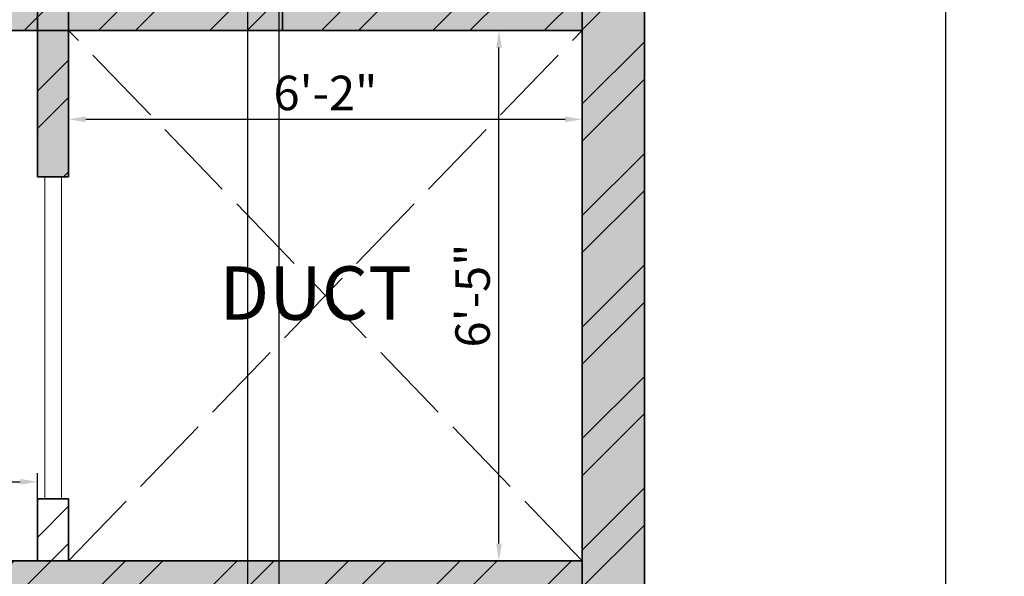
# Model space of a CAD drawing. Units: inches. Extents: x 1804 to 3296, y 909 to 2477.
# Tile 14 of 31: x 2235 to 2378, y 1329 to 1410. Entities that reach past the tile are written whole.
import ezdxf

# ---------------------------------------------------------------- set-up
doc = ezdxf.new("R2010")
doc.units = ezdxf.units.IN
doc.linetypes.add('ACAD_ISO02W100', pattern=[15, 12, -3])
for name, color, linetype, lineweight in [('A-ANNO-DIMS', 2, 'Continuous', 18), ('A-ANNO-TTLB', 156, 'Continuous', 35), ('A-AREA-IDEN', 190, 'Continuous', 18), ('A-FLOR-OPEN', 8, 'ACAD_ISO02W100', 18), ('A-WALL-PATT', 10, 'Continuous', 13), ('WALL', 10, 'Continuous', 35), ('WIND', 130, 'Continuous', 18)]:
    doc.layers.add(name, color=color, linetype=linetype, lineweight=lineweight)
doc.styles.get("Standard").update_dxf_attribs({"font": 'arial.ttf'})
doc.dimstyles.new('ISO-25', dxfattribs={"dimtxt": 5, "dimasz": 2.5, "dimexe": 1.25, "dimexo": 0.625, "dimtad": 1, "dimdec": 0, "dimlunit": 4, "dimtxsty": 'Standard', "dimcen": 2.5, "dimadec": 0, "dimazin": 0, "dimtfac": 1, "dimtdec": 0, "dimtmove": 0, "dimatfit": 3, "dimfxl": 1, "dimarcsym": 0})
pattern_1 = [(45, (0, 196.207), (-8.08223, 8.08223), []), (45, (5.388, 196.207), (-8.08223, 8.08223), [])]

# ---------------------------------------------------------------- blocks, each defined once
blk = doc.blocks.new('*D14')
at = {"layer": 'A-ANNO-DIMS', "color": 0, "lineweight": -2, "transparency": 16777216}
for p, q in [((2242.06, 1407.44), (2242.06, 1393.92)), ((2316.54, 1407.44), (2316.54, 1393.92)), ((2244.56, 1395.17), (2314.04, 1395.17))]:
    blk.add_line(p, q, dxfattribs=at)
at = {"layer": 'A-ANNO-DIMS', "color": 0, "lineweight": 100, "transparency": 16777216}
for points in [[(2244.56, 1395.58), (2244.56, 1394.75), (2242.06, 1395.17)], [(2314.04, 1395.58), (2314.04, 1394.75), (2316.54, 1395.17)]]:
    blk.add_solid(points, dxfattribs=at)
at = {"layer": 'Defpoints', "color": 0, "lineweight": 100, "transparency": 16777216}
for p in [(2242.06, 1408.06), (2316.54, 1408.06), (2316.54, 1395.17)]:
    blk.add_point(p, dxfattribs=at)
at = {"layer": 'A-ANNO-DIMS', "color": 0, "transparency": 16777216, "insert": (2279.3, 1398.34), "char_height": 5, "attachment_point": 5}
blk.add_mtext('6\'-2"', dxfattribs=at)
blk = doc.blocks.new('*D15')
at = {"layer": 'A-ANNO-DIMS', "color": 0, "lineweight": -2, "transparency": 16777216}
for p, q in [((2315.91, 1408.06), (2303.21, 1408.06)), ((2304.46, 1333.69), (2304.46, 1405.56)), ((2315.91, 1331.19), (2303.21, 1331.19))]:
    blk.add_line(p, q, dxfattribs=at)
at = {"layer": 'A-ANNO-DIMS', "color": 0, "lineweight": 100, "transparency": 16777216}
for points in [[(2304.05, 1405.56), (2304.88, 1405.56), (2304.46, 1408.06)], [(2304.05, 1333.69), (2304.88, 1333.69), (2304.46, 1331.19)]]:
    blk.add_solid(points, dxfattribs=at)
at = {"layer": 'Defpoints', "color": 0, "lineweight": 100, "transparency": 16777216}
for p in [(2304.46, 1408.06), (2316.54, 1408.06), (2316.54, 1331.19)]:
    blk.add_point(p, dxfattribs=at)
at = {"layer": 'A-ANNO-DIMS', "color": 0, "transparency": 16777216, "insert": (2301.28, 1369.63), "char_height": 5, "attachment_point": 5, "rotation": 90}
blk.add_mtext('6\'-5"', dxfattribs=at)
blk = doc.blocks.new('*D16')
at = {"layer": 'A-ANNO-DIMS', "color": 0, "lineweight": -2, "transparency": 16777216}
for p, q in [((2158.58, 1331.82), (2158.58, 1343.89)), ((2237.56, 1331.82), (2237.56, 1343.89)), ((2161.08, 1342.64), (2235.06, 1342.64))]:
    blk.add_line(p, q, dxfattribs=at)
at = {"layer": 'A-ANNO-DIMS', "color": 0, "lineweight": 100, "transparency": 16777216}
for points in [[(2161.08, 1343.05), (2161.08, 1342.22), (2158.58, 1342.64)], [(2235.06, 1343.05), (2235.06, 1342.22), (2237.56, 1342.64)]]:
    blk.add_solid(points, dxfattribs=at)
at = {"layer": 'Defpoints', "color": 0, "lineweight": 100, "transparency": 16777216}
for p in [(2237.56, 1342.64), (2158.58, 1331.19), (2237.56, 1331.19)]:
    blk.add_point(p, dxfattribs=at)
at = {"layer": 'A-ANNO-DIMS', "color": 0, "transparency": 16777216, "insert": (2198.07, 1345.81), "char_height": 5, "attachment_point": 5}
blk.add_mtext('6\'-7"', dxfattribs=at)
blk = doc.blocks.new('*D53')
at = {"layer": 'A-ANNO-DIMS', "color": 0, "lineweight": -2, "transparency": 16777216}
for p, q in [((2326.16, 1793.38), (2370.49, 1793.38)), ((2369.24, 1140.57), (2369.24, 1790.88)), ((2326.16, 1138.07), (2370.49, 1138.07))]:
    blk.add_line(p, q, dxfattribs=at)
at = {"layer": 'A-ANNO-DIMS', "color": 0, "lineweight": 100, "transparency": 16777216}
for points in [[(2368.82, 1790.88), (2369.65, 1790.88), (2369.24, 1793.38)], [(2368.82, 1140.57), (2369.65, 1140.57), (2369.24, 1138.07)]]:
    blk.add_solid(points, dxfattribs=at)
at = {"layer": 'Defpoints', "color": 0, "lineweight": 100, "transparency": 16777216}
for p in [(2325.54, 1793.38), (2369.24, 1793.38), (2325.54, 1138.07)]:
    blk.add_point(p, dxfattribs=at)
at = {"layer": 'A-ANNO-DIMS', "color": 0, "transparency": 16777216, "insert": (2366.03, 1465.72), "char_height": 5, "attachment_point": 5, "rotation": 90}
blk.add_mtext('54\'-7 1/2"', dxfattribs=at)
blk = doc.blocks.new('*D56')
at = {"layer": 'A-ANNO-DIMS', "color": 0, "lineweight": -2, "transparency": 16777216}
for p, q in [((2180.87, 1680.42), (2180.87, 975.89)), ((2268, 1680.42), (2268, 975.89)), ((2183.37, 977.14), (2265.5, 977.14))]:
    blk.add_line(p, q, dxfattribs=at)
at = {"layer": 'A-ANNO-DIMS', "color": 0, "lineweight": 100, "transparency": 16777216}
for points in [[(2183.37, 977.56), (2183.37, 976.72), (2180.87, 977.14)], [(2265.5, 977.56), (2265.5, 976.72), (2268, 977.14)]]:
    blk.add_solid(points, dxfattribs=at)
at = {"layer": 'Defpoints', "color": 0, "lineweight": 100, "transparency": 16777216}
for p in [(2180.87, 1681.04), (2268, 1681.04), (2268, 977.14)]:
    blk.add_point(p, dxfattribs=at)
at = {"layer": 'A-ANNO-DIMS', "color": 0, "transparency": 16777216, "insert": (2224.44, 980.32), "char_height": 5, "attachment_point": 5}
blk.add_mtext('7\'-3"', dxfattribs=at)
blk = doc.blocks.new('*D73')
at = {"layer": 'A-ANNO-DIMS', "color": 0, "lineweight": -2, "transparency": 16777216}
for p, q in [((2272.59, 1272.26), (2272.59, 1874.99)), ((2316.54, 1272.26), (2316.54, 1874.99)), ((2275.09, 1873.74), (2314.04, 1873.74))]:
    blk.add_line(p, q, dxfattribs=at)
at = {"layer": 'A-ANNO-DIMS', "color": 0, "lineweight": 100, "transparency": 16777216}
for points in [[(2275.09, 1874.15), (2275.09, 1873.32), (2272.59, 1873.74)], [(2314.04, 1874.15), (2314.04, 1873.32), (2316.54, 1873.74)]]:
    blk.add_solid(points, dxfattribs=at)
at = {"layer": 'Defpoints', "color": 0, "lineweight": 100, "transparency": 16777216}
for p in [(2316.54, 1873.74), (2272.59, 1271.63), (2316.54, 1271.63)]:
    blk.add_point(p, dxfattribs=at)
at = {"layer": 'A-ANNO-DIMS', "color": 0, "transparency": 16777216, "insert": (2294.56, 1876.92), "char_height": 5, "attachment_point": 5}
blk.add_mtext('3\'-8"', dxfattribs=at)

msp = doc.modelspace()

# ---------------------------------------------------------------- hatches: boundary and pattern name
at = {"layer": 'A-ANNO-TTLB'}
h = msp.add_hatch(color=256, dxfattribs=at)
h.dxf.hatch_style = 1
h.paths.add_polyline_path([(3294.53, 2476.54), (1803.79, 2476.54), (1805.43, 909.47), (3296.17, 909.47)])
h.paths.add_polyline_path([(1811, 914.33), (1812.79, 2467.54), (3285.53, 2467.54), (3283.74, 914.33)], flags=16)
h.paths.add_polyline_path([(1925.58, 1062.77), (1925.58, 1138.07), (1925.58, 1539.88), (1925.58, 1793.38), (1925.58, 1830.04), (2325.54, 1830.04), (2325.54, 1793.38), (2325.54, 1586.42), (2325.54, 1138.07), (2325.54, 1062.77)], flags=0)
h.paths.add_polyline_path([(1997.22, 1029.4), (2008.85, 1037.96), (2008.85, 1020.84)], flags=0)
h.paths.add_polyline_path([(1934.58, 1138.07), (1934.58, 1147.07), (2078.77, 1147.07), (2078.77, 1138.07), (2060.94, 1138.07)], flags=0)
h.paths.add_polyline_path([(1944.35, 1138.07), (1944.35, 1147.07), (2056.05, 1147.07), (2056.05, 1138.07)], flags=0)
h.paths.add_polyline_path([(2222.24, 1037.96), (2233.87, 1029.4), (2222.24, 1020.84)], flags=0)
h.paths.add_polyline_path([(2061.94, 1139.07), (2061.94, 1146.07), (2077.77, 1146.07), (2077.77, 1139.07)], flags=0)
h.paths.add_polyline_path([(2149.58, 1138.07), (2149.58, 1269.44), (2158.58, 1269.44), (2158.58, 1326.69), (2149.58, 1326.69), (2149.58, 1340.94), (2139.6, 1340.94), (2139.6, 1434.25), (2149.58, 1434.25), (2149.58, 1447.36), (2158.58, 1447.36), (2158.58, 1423.87), (2158.58, 1408.06), (2198.46, 1408.06), (2198.46, 1412.56), (2282.65, 1412.56), (2282.65, 1465.94), (2316.54, 1465.94), (2316.54, 1590.92), (2192.86, 1590.92), (2192.86, 1595.3), (2291.17, 1595.3), (2291.17, 1590.92), (2316.54, 1590.92), (2316.54, 1784.38), (2300.24, 1784.38), (2300.24, 1757.47), (2268, 1757.47), (2268, 1681.04), (2180.87, 1681.04), (2180.87, 1757.47), (2148.63, 1757.47), (2148.63, 1784.38), (2119.08, 1784.38), (2119.08, 1585.58), (2114.58, 1585.58), (2114.58, 1784.38), (2064.11, 1784.38), (2046.28, 1784.38), (2046.28, 1760.38), (1958.58, 1760.38), (1958.58, 1664.38), (1934.58, 1664.38), (1934.58, 1784.38), (1934.58, 1793.38), (2046.28, 1793.38), (2064.11, 1793.38), (2119.08, 1793.38), (2230.78, 1793.38), (2230.78, 1784.38), (2268, 1784.38), (2300.24, 1784.38), (2316.54, 1784.38), (2316.54, 1590.92), (2316.54, 1373.73), (2316.54, 1138.07)], flags=0)
h.paths.add_polyline_path([(2209.19, 1166.63), (2209.19, 1175.63), (2158.58, 1175.63), (2209.19, 1223.63), (2209.19, 1231.63), (2183.88, 1231.63), (2183.88, 1301.66), (2242.59, 1301.66), (2242.59, 1326.69), (2316.54, 1326.69), (2272.59, 1271.63), (2272.59, 1223.63), (2316.54, 1175.63), (2272.59, 1175.63), (2272.59, 1166.63)], flags=0)
h.paths.add_polyline_path([(1947.77, 1345.22), (1947.77, 1457.48), (1991.2, 1457.48), (1991.2, 1451.7), (1991.2, 1352.18), (1991.2, 1345.22)], flags=0)
h.paths.add_polyline_path([(2209.19, 1271.63), (2262.59, 1271.63), (2262.59, 1311.85), (2272.59, 1301.66), (2272.59, 1271.63), (2269.92, 1269.63), (2270.59, 1269.63), (2270.59, 1225.63), (2211.19, 1225.63), (2211.19, 1269.63), (2211.86, 1269.63)], flags=0)
h.paths.add_polyline_path([(2000.34, 1378.21), (2000.34, 1429.71), (2025.22, 1429.71), (2025.22, 1378.21)], flags=0)
h.paths.add_polyline_path([(2001.34, 1379.21), (2001.34, 1428.71), (2024.22, 1428.71), (2024.22, 1379.21)], flags=0)
h.paths.add_polyline_path([(2012.34, 1390.21), (2012.34, 1417.71), (2013.22, 1417.71), (2013.22, 1390.21)], flags=0)
h.paths.add_polyline_path([(2237.56, 1331.19), (2237.56, 1340.18), (2238.62, 1340.18), (2238.62, 1386.84), (2241.04, 1386.84), (2242.06, 1386.84), (2242.06, 1408.06), (2316.54, 1331.19)], flags=0)
h.paths.add_polyline_path([(1953.73, 1464.35), (1953.73, 1498.59), (1981.74, 1498.59), (1981.74, 1464.35)], flags=0)
h.paths.add_polyline_path([(1987.63, 1462.08), (1987.63, 1500.95), (2104.07, 1500.95), (2104.07, 1462.08), (2099.27, 1462.08), (1993.6, 1462.08)], flags=0)
h.paths.add_polyline_path([(1956.06, 1481.47, -1), (1979.41, 1481.47, -1)], flags=0)
edge = h.paths.add_edge_path(flags=0)
edge.add_ellipse((2299.53, 1438.37), major_axis=(0.31, 21.36), ratio=0.670333, start_angle=0, end_angle=360)
h.paths.add_polyline_path([(2297.39, 1438.37, -1), (2301.67, 1438.37, -1)], flags=0)
h.paths.add_polyline_path([(2591.54, 1163.23), (2591.54, 1179.38), (2591.54, 1379.68), (2591.54, 1395.84), (2734.5, 1395.84), (2734.5, 1379.68), (2734.5, 1179.38), (2734.5, 1163.23)], flags=0)
h.paths.add_polyline_path([(2592.54, 1164.23), (2592.54, 1166.23), (2733.5, 1166.23), (2733.5, 1164.23)], flags=0)
h.paths.add_polyline_path([(2592.54, 1180.38), (2592.54, 1378.68), (2733.5, 1378.68), (2733.5, 1180.38)], flags=0)
h.paths.add_polyline_path([(2593.54, 1181.38), (2593.54, 1377.68), (2732.5, 1377.68), (2732.5, 1181.38)], flags=0)
h.paths.add_polyline_path([(2594.54, 1182.38), (2594.54, 1376.68), (2731.5, 1376.68), (2731.5, 1182.38)], flags=0)
h.paths.add_polyline_path([(1936.95, 1697.46), (1936.95, 1736.46), (1955.41, 1736.46), (1955.41, 1697.46)], flags=0)
h.paths.add_polyline_path([(1938.48, 1718.36), (1938.48, 1734.92), (1953.65, 1734.92), (1953.65, 1718.36)], flags=0)
h.paths.add_polyline_path([(1944.75, 1726.64, -1), (1947.37, 1726.64, -1)], flags=0)
h.paths.add_polyline_path([(2592.54, 1394.84), (2733.5, 1394.84), (2733.5, 1392.84), (2592.54, 1392.84)], flags=0)
h.paths.add_polyline_path([(1976.61, 1762.5), (1976.61, 1781.44), (2012.79, 1781.44), (2012.79, 1762.5)], flags=0)
h.paths.add_polyline_path([(1979.57, 1771.97, -1), (1991.39, 1771.97, -1)], flags=0)
h.paths.add_polyline_path([(1995.36, 1771.97, -1), (2007.18, 1771.97, -1)], flags=0)
h.paths.add_polyline_path([(2251.51, 1744.53), (2268, 1730.05), (2251.51, 1730.05)], flags=0)
h.paths.add_polyline_path([(2047.28, 1785.38), (2047.28, 1792.38), (2063.11, 1792.38), (2063.11, 1785.38)], flags=0)
h.paths.add_polyline_path([(2155.08, 1770.92, -1), (2174.42, 1770.92, -1)], flags=0)
h.paths.add_polyline_path([(2188.59, 1758.27), (2188.59, 1772.81), (2222.3, 1772.81), (2222.3, 1758.27)], flags=0)
h.paths.add_polyline_path([(2223.97, 1758.27), (2223.97, 1772.81), (2257.68, 1772.81), (2257.68, 1758.27)], flags=0)
h.paths.add_polyline_path([(2274.45, 1770.92, -1), (2293.8, 1770.92, -1)], flags=0)
h.paths.add_polyline_path([(2591.54, 1582.09), (2591.54, 1782.39), (2734.5, 1782.39), (2734.5, 1582.09)], flags=0)
h.paths.add_polyline_path([(2592.54, 1583.09), (2592.54, 1781.39), (2733.5, 1781.39), (2733.5, 1583.09)], flags=0)
h.paths.add_polyline_path([(2593.54, 1584.09), (2593.54, 1780.39), (2732.5, 1780.39), (2732.5, 1584.09)], flags=0)
h.paths.add_polyline_path([(2594.54, 1585.09), (2594.54, 1779.39), (2731.5, 1779.39), (2731.5, 1585.09)], flags=0)
h.paths.add_polyline_path([(1922.17, 1978.79), (1922.17, 2295.08), (1922.17, 2296.08), (2115.67, 2296.08), (2115.67, 2384.31), (2115.67, 2385.31), (2322.12, 2385.31), (2323.12, 2385.31), (2323.12, 1979.79), (2323.12, 1978.79), (1923.17, 1978.79)], flags=0)
h.paths.add_polyline_path([(1922.17, 1978.79), (1922.17, 2051.31), (1922.17, 2214.86), (1922.17, 2296.08), (2115.67, 2296.08), (2115.67, 2385.31), (2323.12, 2385.31), (2323.12, 2280.42), (2323.12, 1978.79), (2115.67, 1978.79)], flags=0)
h.paths.add_polyline_path([(1923.17, 1979.79), (1923.17, 2050.31), (2115.67, 2050.31), (2115.67, 2051.31), (1923.17, 2051.31), (1923.17, 2213.86), (1923.17, 2214.86), (1923.17, 2295.08), (1990.02, 2295.08), (1990.02, 2214.86), (1991.02, 2214.86), (1991.02, 2295.08), (2115.67, 2295.08), (2115.67, 1979.79), (2116.67, 1979.79), (2116.67, 2304.18), (2116.67, 2384.31), (2322.12, 2384.31), (2322.12, 2280.42), (2322.12, 1979.79), (2115.67, 1979.79)], flags=0)
h.paths.add_polyline_path([(2972.46, 1192.5), (2972.46, 1196.92), (2995.47, 1196.92), (2995.47, 1255.47), (2995.09, 1255.47), (2987.42, 1249.39), (2980.08, 1255.47), (2978.05, 1255.47), (2978.05, 1257.24), (2995.47, 1257.24), (2995.47, 1261.58), (3015.37, 1261.58), (3015.37, 1333.28), (3015.37, 1414.4), (3032.82, 1414.4), (3032.82, 1333.28), (3032.82, 1261.58), (3052.66, 1261.58), (3052.66, 1255.47), (3079.86, 1255.47), (3078.72, 1254.57), (3081.47, 1252.29), (3078.56, 1249.99), (3075.81, 1252.26), (3072.57, 1249.69), (3070.36, 1251.52), (3067.67, 1249.39), (3060.34, 1255.47), (3052.66, 1255.47), (3052.66, 1196.92), (3054.58, 1196.92), (3074, 1196.92), (3074, 1192.5), (3052.66, 1192.5), (2995.47, 1192.5)], flags=0)
h.paths.add_polyline_path([(2490.75, 1979.27), (2490.75, 1980.27), (2596.87, 1980.27), (2596.87, 2051.8), (2596.87, 2052.8), (2596.87, 2216.35), (2596.87, 2297.57), (2717.32, 2297.57), (2710.57, 2305.62), (2724.07, 2305.62), (2717.32, 2297.57), (2782.37, 2297.57), (2782.37, 2395.8), (3006.82, 2395.8), (3006.82, 1981.27), (3093.73, 1981.27), (3093.73, 1980.27), (3047.51, 1980.27), (3046.37, 1979.37), (3049.11, 1977.1), (3046.2, 1974.79), (3043.46, 1977.07), (3040.21, 1974.49), (3038, 1976.32), (3035.32, 1974.2), (3027.98, 1980.27), (2871.83, 1980.27), (2871.83, 1981.27), (2791.37, 1981.27), (2791.37, 2050.8), (2597.87, 2050.8), (2597.87, 1980.27), (2597.87, 1979.27), (2546.27, 1979.27), (2545.12, 1978.37), (2547.87, 1976.1), (2544.96, 1973.79), (2542.22, 1976.07), (2538.97, 1973.49), (2536.76, 1975.32), (2534.07, 1973.2), (2526.74, 1979.27)], flags=0)
h.paths.add_polyline_path([(2597.87, 2051.8), (2606.87, 2051.8), (2606.87, 2258.39), (2597.87, 2258.39), (2597.87, 2296.57), (2606.87, 2296.57), (2606.87, 2262.39), (2782.37, 2262.39), (2782.37, 2296.57), (2790.37, 2296.57), (2790.37, 2262.39), (2791.37, 2262.39), (2791.37, 2305.67), (2791.37, 2385.8), (2996.82, 2385.8), (2996.82, 2339.85), (3006.82, 2339.85), (3006.82, 2250.12), (2997.82, 2250.12), (2997.82, 1981.27), (2996.82, 1981.27), (2872.83, 1981.27), (2872.83, 1991.8), (2871.83, 1991.8), (2871.83, 2050.8), (2790.37, 2050.8), (2597.87, 2050.8)], flags=0)
h.paths.add_polyline_path([(2179.93, 2153.92), (2179.93, 2353.97), (2259.98, 2353.97), (2259.98, 2153.92)], flags=0)
h.paths.add_polyline_path([(2180.93, 2154.92), (2180.93, 2352.97), (2258.98, 2352.97), (2258.98, 2154.92)], flags=0)
h.paths.add_polyline_path([(2960.87, 1608.49), (2960.87, 1753.62), (3070.9, 1753.62), (3070.9, 1608.49)], flags=0)
h.paths.add_polyline_path([(2961.87, 1609.49), (2961.87, 1752.62), (3069.9, 1752.62), (3069.9, 1609.49)], flags=0)
h.paths.add_polyline_path([(2962.87, 1610.49), (2962.87, 1751.62), (3068.9, 1751.62), (3068.9, 1610.49)], flags=0)
h.paths.add_polyline_path([(2963.87, 1611.49), (2963.87, 1750.62), (3067.9, 1750.62), (3067.9, 1611.49)], flags=0)
h.paths.add_polyline_path([(2782.37, 2051.8), (2782.37, 2216.32), (2791.37, 2216.32), (2791.37, 2051.8), (2872.83, 2051.8), (2872.83, 2068.56), (2884.67, 2068.56), (2884.67, 2085.33), (2896.51, 2085.33), (2896.51, 2102.09), (2908.36, 2102.09), (2908.36, 2118.85), (2920.2, 2118.85), (2920.2, 2135.62), (2932.05, 2135.62), (2932.05, 2145.3), (2925.08, 2145.3), (2925.08, 2203.2), (2996.82, 2203.2), (2996.82, 2145.3), (2953.82, 2145.3), (2872.83, 2051.8), (2790.37, 2051.8)], flags=0)
h.paths.add_polyline_path([(2717.32, 2238.65), (2710.57, 2246.7), (2724.07, 2246.7)], flags=0)
h.paths.add_polyline_path([(2003.09, 1122.79), (2017.16, 1122.79), (2017.16, 1138.74), (2003.09, 1138.74)], flags=8)
h.paths.add_polyline_path([(2174.76, 1792.72), (2188.83, 1792.72), (2188.83, 1808.66), (2174.76, 1808.66)], flags=8)
h.paths.add_polyline_path([(1987.95, 1792.51), (2002.02, 1792.51), (2002.02, 1808.45), (1987.95, 1808.45)], flags=8)
h.paths.add_polyline_path([(2148.79, 1289.26), (2160.46, 1289.26), (2160.46, 1305.2), (2148.79, 1305.2)], flags=8)
h.paths.add_polyline_path([(2115.36, 1133.57), (2127.04, 1133.57), (2127.04, 1149.51), (2115.36, 1149.51)], flags=8)
h.paths.add_polyline_path([(2237.58, 1421.48), (2249.25, 1421.48), (2249.25, 1437.43), (2237.58, 1437.43)], flags=8)
h.paths.add_polyline_path([(2134.99, 1584.32), (2146.66, 1584.32), (2146.66, 1600.26), (2134.99, 1600.26)], flags=8)
h.paths.add_polyline_path([(2101.95, 1557.31), (2113.62, 1557.31), (2113.62, 1573.25), (2101.95, 1573.25)], flags=8)
h.paths.add_polyline_path([(2937.85, 1156.77), (3120.41, 1156.77), (3120.41, 1185.72), (2937.85, 1185.72)], flags=8)
h.paths.add_polyline_path([(2980.71, 1786.71), (3050.06, 1786.71), (3050.06, 1802.66), (2980.71, 1802.66)], flags=8)
h.paths.add_polyline_path([(2869.28, 1661.96), (2938.62, 1661.96), (2938.62, 1690.8), (2869.28, 1690.8)], flags=8)
h.paths.add_polyline_path([(3092.27, 1674.86), (3161.62, 1674.86), (3161.62, 1690.8), (3092.27, 1690.8)], flags=8)
h.paths.add_polyline_path([(2980.71, 1674.86), (3050.06, 1674.86), (3050.06, 1690.8), (2980.71, 1690.8)], flags=8)
h.paths.add_polyline_path([(2649.07, 1678.23), (2674.53, 1678.23), (2674.53, 1714.76), (2649.07, 1714.76)], flags=8)
h.paths.add_polyline_path([(2530.84, 1981.63), (2549.13, 1981.63), (2549.13, 1997.57), (2530.84, 1997.57)], flags=8)
h.paths.add_polyline_path([(3031.29, 1981.77), (3049.58, 1981.77), (3049.58, 1997.71), (3031.29, 1997.71)], flags=8)
h.paths.add_polyline_path([(2715.38, 1911.9), (2851.54, 1911.9), (2851.54, 1940.85), (2715.38, 1940.85)], flags=8)
h.paths.add_polyline_path([(2015.23, 1927.36), (2205.42, 1927.36), (2205.42, 1956.3), (2015.23, 1956.3)], flags=8)
h.paths.add_polyline_path([(2671.84, 2057.84), (2702.75, 2057.84), (2702.75, 2073.79), (2671.84, 2073.79)], flags=8)
h.paths.add_polyline_path([(2678.5, 2316.52), (2765.26, 2316.52), (2765.26, 2332.46), (2678.5, 2332.46)], flags=8)
h.paths.add_polyline_path([(2678.48, 2271.96), (2736.41, 2271.96), (2736.41, 2287.9), (2678.48, 2287.9)], flags=8)
h.paths.add_polyline_path([(2019.2, 972.79), (2243.21, 972.79), (2243.21, 1001.74), (2019.2, 1001.74)], flags=8)
h.paths.add_polyline_path([(2097.06, 1021.56), (2132.16, 1021.56), (2132.16, 1037.51), (2097.06, 1037.51)], flags=8)
h.paths.add_polyline_path([(2182.47, 1360.48), (2207.35, 1360.48), (2207.35, 1376.42), (2182.47, 1376.42)], flags=8)
h.paths.add_polyline_path([(2261.12, 1361.77), (2295.01, 1361.77), (2295.01, 1377.71), (2261.12, 1377.71)], flags=8)
h.paths.add_polyline_path([(2245.75, 1511.51), (2278.44, 1511.51), (2278.44, 1527.46), (2245.75, 1527.46)], flags=8)
h.paths.add_polyline_path([(1991.16, 1296.29), (2060.51, 1296.29), (2060.51, 1312.23), (1991.16, 1312.23)], flags=8)
h.paths.add_polyline_path([(2187, 1651.35), (2246.71, 1651.35), (2246.71, 1667.29), (2187, 1667.29)], flags=8)
h.paths.add_polyline_path([(1976.49, 1684.81), (2068.63, 1684.81), (2068.63, 1700.76), (1976.49, 1700.76)], flags=8)
at = {"layer": 'A-WALL-PATT'}
h = msp.add_hatch(color=256, dxfattribs=at)
h.dxf.hatch_style = 1
h.paths.add_polyline_path([(2119.08, 1544.38), (1925.58, 1544.38), (1925.58, 1539.88), (2119.08, 1539.88)])
h.paths.add_polyline_path([(2119.08, 1545.58), (2114.58, 1545.58), (2114.58, 1544.38), (2119.08, 1544.38)])
h.paths.add_polyline_path([(1965.87, 1658.79), (1965.87, 1679.09), (1955.57, 1679.09), (1955.57, 1658.79)], flags=9)
h.paths.add_polyline_path([(2293.18, 1677.29), (2293.18, 1697.58), (2282.88, 1697.58), (2282.88, 1677.29)], flags=9)
h.paths.add_polyline_path([(2271.13, 1545.23), (2287.53, 1545.23), (2287.53, 1555.53), (2271.13, 1555.53)], flags=9)
h.paths.add_polyline_path([(2303.26, 1488.52), (2303.26, 1508.82), (2292.95, 1508.82), (2292.95, 1488.52)], flags=9)
h.paths.add_polyline_path([(2271.13, 1393.15), (2287.53, 1393.15), (2287.53, 1403.45), (2271.13, 1403.45)], flags=9)
h.paths.add_polyline_path([(2306.48, 1361.45), (2306.48, 1377.86), (2296.18, 1377.86), (2296.18, 1361.45)], flags=9)
h.paths.add_polyline_path([(2174.54, 1361.45), (2174.54, 1377.86), (2164.23, 1377.86), (2164.23, 1361.45)], flags=9)
h.paths.add_polyline_path([(1968.21, 1333.34), (1968.21, 1353.64), (1957.91, 1353.64), (1957.91, 1333.34)], flags=9)
h.paths.add_polyline_path([(2003.09, 1122.79), (2017.16, 1122.79), (2017.16, 1138.74), (2003.09, 1138.74)], flags=9)
h.paths.add_polyline_path([(2174.76, 1792.72), (2188.83, 1792.72), (2188.83, 1808.66), (2174.76, 1808.66)], flags=9)
h.paths.add_polyline_path([(1987.95, 1792.51), (2002.02, 1792.51), (2002.02, 1808.45), (1987.95, 1808.45)], flags=9)
h.paths.add_polyline_path([(2148.79, 1289.26), (2160.46, 1289.26), (2160.46, 1305.2), (2148.79, 1305.2)], flags=9)
h.paths.add_polyline_path([(2115.36, 1133.57), (2127.04, 1133.57), (2127.04, 1149.51), (2115.36, 1149.51)], flags=9)
h.paths.add_polyline_path([(2237.58, 1421.48), (2249.25, 1421.48), (2249.25, 1437.43), (2237.58, 1437.43)], flags=9)
h.paths.add_polyline_path([(2134.99, 1584.32), (2146.66, 1584.32), (2146.66, 1600.26), (2134.99, 1600.26)], flags=9)
h.paths.add_polyline_path([(2101.95, 1557.31), (2113.62, 1557.31), (2113.62, 1573.25), (2101.95, 1573.25)], flags=9)
h.paths.add_polyline_path([(2937.85, 1156.77), (3120.41, 1156.77), (3120.41, 1185.72), (2937.85, 1185.72)], flags=9)
h.paths.add_polyline_path([(2980.71, 1786.71), (3050.06, 1786.71), (3050.06, 1802.66), (2980.71, 1802.66)], flags=9)
h.paths.add_polyline_path([(2869.28, 1661.96), (2938.62, 1661.96), (2938.62, 1690.8), (2869.28, 1690.8)], flags=9)
h.paths.add_polyline_path([(3092.27, 1674.86), (3161.62, 1674.86), (3161.62, 1690.8), (3092.27, 1690.8)], flags=9)
h.paths.add_polyline_path([(2980.71, 1674.86), (3050.06, 1674.86), (3050.06, 1690.8), (2980.71, 1690.8)], flags=9)
h.paths.add_polyline_path([(2649.07, 1678.23), (2674.53, 1678.23), (2674.53, 1714.76), (2649.07, 1714.76)], flags=9)
h.paths.add_polyline_path([(2530.84, 1981.63), (2549.13, 1981.63), (2549.13, 1997.57), (2530.84, 1997.57)], flags=9)
h.paths.add_polyline_path([(3031.29, 1981.77), (3049.58, 1981.77), (3049.58, 1997.71), (3031.29, 1997.71)], flags=9)
h.paths.add_polyline_path([(2715.38, 1911.9), (2851.54, 1911.9), (2851.54, 1940.85), (2715.38, 1940.85)], flags=9)
h.paths.add_polyline_path([(2015.23, 1927.36), (2205.42, 1927.36), (2205.42, 1956.3), (2015.23, 1956.3)], flags=9)
h.paths.add_polyline_path([(2671.84, 2057.84), (2702.75, 2057.84), (2702.75, 2073.79), (2671.84, 2073.79)], flags=9)
h.paths.add_polyline_path([(2678.5, 2316.52), (2765.26, 2316.52), (2765.26, 2332.46), (2678.5, 2332.46)], flags=9)
h.paths.add_polyline_path([(2678.48, 2271.96), (2736.41, 2271.96), (2736.41, 2287.9), (2678.48, 2287.9)], flags=9)
h.paths.add_polyline_path([(2019.2, 972.79), (2243.21, 972.79), (2243.21, 1001.74), (2019.2, 1001.74)], flags=9)
h.paths.add_polyline_path([(2097.06, 1021.56), (2132.16, 1021.56), (2132.16, 1037.51), (2097.06, 1037.51)], flags=9)
h.paths.add_polyline_path([(2182.47, 1360.48), (2207.35, 1360.48), (2207.35, 1376.42), (2182.47, 1376.42)], flags=9)
h.paths.add_polyline_path([(2261.12, 1361.77), (2295.01, 1361.77), (2295.01, 1377.71), (2261.12, 1377.71)], flags=9)
h.paths.add_polyline_path([(2245.75, 1511.51), (2278.44, 1511.51), (2278.44, 1527.46), (2245.75, 1527.46)], flags=9)
h.paths.add_polyline_path([(1991.16, 1296.29), (2060.51, 1296.29), (2060.51, 1312.23), (1991.16, 1312.23)], flags=9)
h.paths.add_polyline_path([(2187, 1651.35), (2246.71, 1651.35), (2246.71, 1667.29), (2187, 1667.29)], flags=9)
h.paths.add_polyline_path([(1976.49, 1684.81), (2068.63, 1684.81), (2068.63, 1700.76), (1976.49, 1700.76)], flags=9)
h = msp.add_hatch(color=256, dxfattribs=at)
h.dxf.hatch_style = 1
h.paths.add_polyline_path([(2149.58, 1147.07), (2141.21, 1147.07), (2141.21, 1144.07), (2141.21, 1138.07), (2149.58, 1138.07)])
h.paths.add_polyline_path([(2101.21, 1144.07, -0.01877), (2101.32, 1147.07), (2078.77, 1147.07), (2078.77, 1138.07), (2101.21, 1138.07)])
h.paths.add_polyline_path([(2060.94, 1147.07), (2056.05, 1147.07), (2056.05, 1138.07), (2060.94, 1138.07)])
h.paths.add_polyline_path([(1944.35, 1147.07), (1934.58, 1147.07), (1934.58, 1138.07), (1944.35, 1138.07)])
h.paths.add_polyline_path([(2158.58, 1269.44), (2149.58, 1269.44), (2149.58, 1138.07), (2158.58, 1138.07)])
h.paths.add_polyline_path([(2003.09, 1122.79), (2017.16, 1122.79), (2017.16, 1138.74), (2003.09, 1138.74)], flags=9)
h.paths.add_polyline_path([(2174.76, 1792.72), (2188.83, 1792.72), (2188.83, 1808.66), (2174.76, 1808.66)], flags=9)
h.paths.add_polyline_path([(1987.95, 1792.51), (2002.02, 1792.51), (2002.02, 1808.45), (1987.95, 1808.45)], flags=9)
h.paths.add_polyline_path([(2148.79, 1289.26), (2160.46, 1289.26), (2160.46, 1305.2), (2148.79, 1305.2)], flags=9)
h.paths.add_polyline_path([(2115.36, 1133.57), (2127.04, 1133.57), (2127.04, 1149.51), (2115.36, 1149.51)], flags=9)
h.paths.add_polyline_path([(2237.58, 1421.48), (2249.25, 1421.48), (2249.25, 1437.43), (2237.58, 1437.43)], flags=9)
h.paths.add_polyline_path([(2134.99, 1584.32), (2146.66, 1584.32), (2146.66, 1600.26), (2134.99, 1600.26)], flags=9)
h.paths.add_polyline_path([(2101.95, 1557.31), (2113.62, 1557.31), (2113.62, 1573.25), (2101.95, 1573.25)], flags=9)
h.paths.add_polyline_path([(2937.85, 1156.77), (3120.41, 1156.77), (3120.41, 1185.72), (2937.85, 1185.72)], flags=9)
h.paths.add_polyline_path([(2980.71, 1786.71), (3050.06, 1786.71), (3050.06, 1802.66), (2980.71, 1802.66)], flags=9)
h.paths.add_polyline_path([(2869.28, 1661.96), (2938.62, 1661.96), (2938.62, 1690.8), (2869.28, 1690.8)], flags=9)
h.paths.add_polyline_path([(3092.27, 1674.86), (3161.62, 1674.86), (3161.62, 1690.8), (3092.27, 1690.8)], flags=9)
h.paths.add_polyline_path([(2980.71, 1674.86), (3050.06, 1674.86), (3050.06, 1690.8), (2980.71, 1690.8)], flags=9)
h.paths.add_polyline_path([(2649.07, 1678.23), (2674.53, 1678.23), (2674.53, 1714.76), (2649.07, 1714.76)], flags=9)
h.paths.add_polyline_path([(2530.84, 1981.63), (2549.13, 1981.63), (2549.13, 1997.57), (2530.84, 1997.57)], flags=9)
h.paths.add_polyline_path([(3031.29, 1981.77), (3049.58, 1981.77), (3049.58, 1997.71), (3031.29, 1997.71)], flags=9)
h.paths.add_polyline_path([(2715.38, 1911.9), (2851.54, 1911.9), (2851.54, 1940.85), (2715.38, 1940.85)], flags=9)
h.paths.add_polyline_path([(2015.23, 1927.36), (2205.42, 1927.36), (2205.42, 1956.3), (2015.23, 1956.3)], flags=9)
h.paths.add_polyline_path([(2671.84, 2057.84), (2702.75, 2057.84), (2702.75, 2073.79), (2671.84, 2073.79)], flags=9)
h.paths.add_polyline_path([(2678.5, 2316.52), (2765.26, 2316.52), (2765.26, 2332.46), (2678.5, 2332.46)], flags=9)
h.paths.add_polyline_path([(2678.48, 2271.96), (2736.41, 2271.96), (2736.41, 2287.9), (2678.48, 2287.9)], flags=9)
h.paths.add_polyline_path([(2019.2, 972.79), (2243.21, 972.79), (2243.21, 1001.74), (2019.2, 1001.74)], flags=9)
h.paths.add_polyline_path([(2097.06, 1021.56), (2132.16, 1021.56), (2132.16, 1037.51), (2097.06, 1037.51)], flags=9)
h.paths.add_polyline_path([(2182.47, 1360.48), (2207.35, 1360.48), (2207.35, 1376.42), (2182.47, 1376.42)], flags=9)
h.paths.add_polyline_path([(2261.12, 1361.77), (2295.01, 1361.77), (2295.01, 1377.71), (2261.12, 1377.71)], flags=9)
h.paths.add_polyline_path([(2245.75, 1511.51), (2278.44, 1511.51), (2278.44, 1527.46), (2245.75, 1527.46)], flags=9)
h.paths.add_polyline_path([(1991.16, 1296.29), (2060.51, 1296.29), (2060.51, 1312.23), (1991.16, 1312.23)], flags=9)
h.paths.add_polyline_path([(2187, 1651.35), (2246.71, 1651.35), (2246.71, 1667.29), (2187, 1667.29)], flags=9)
h.paths.add_polyline_path([(1976.49, 1684.81), (2068.63, 1684.81), (2068.63, 1700.76), (1976.49, 1700.76)], flags=9)
h = msp.add_hatch(color=256, dxfattribs=at)
h.dxf.hatch_style = 1
h.paths.add_polyline_path([(2158.58, 1275.49), (2155.29, 1275.49), (2149.58, 1275.49), (2149.58, 1269.44), (2158.58, 1269.44)])
h.paths.add_polyline_path([(2158.58, 1326.69), (2149.58, 1326.69), (2149.58, 1319.33), (2155.29, 1319.33), (2158.58, 1319.33)])
h.paths.add_polyline_path([(2158.58, 1402.2), (2158.58, 1423.87), (2158.58, 1447.36), (2149.58, 1447.36), (2149.58, 1423.87), (2149.58, 1340.94), (2149.58, 1326.69), (2158.58, 1326.69), (2158.58, 1354.23)])
h.paths.add_polyline_path([(1965.87, 1658.79), (1965.87, 1679.09), (1955.57, 1679.09), (1955.57, 1658.79)], flags=9)
h.paths.add_polyline_path([(2293.18, 1677.29), (2293.18, 1697.58), (2282.88, 1697.58), (2282.88, 1677.29)], flags=9)
h.paths.add_polyline_path([(2271.13, 1545.23), (2287.53, 1545.23), (2287.53, 1555.53), (2271.13, 1555.53)], flags=9)
h.paths.add_polyline_path([(2303.26, 1488.52), (2303.26, 1508.82), (2292.95, 1508.82), (2292.95, 1488.52)], flags=9)
h.paths.add_polyline_path([(2271.13, 1393.15), (2287.53, 1393.15), (2287.53, 1403.45), (2271.13, 1403.45)], flags=9)
h.paths.add_polyline_path([(2306.48, 1361.45), (2306.48, 1377.86), (2296.18, 1377.86), (2296.18, 1361.45)], flags=9)
h.paths.add_polyline_path([(2189.9, 1340.62), (2206.31, 1340.62), (2206.31, 1350.92), (2189.9, 1350.92)], flags=9)
h.paths.add_polyline_path([(2174.54, 1361.45), (2174.54, 1377.86), (2164.23, 1377.86), (2164.23, 1361.45)], flags=9)
h.paths.add_polyline_path([(2304.24, 1240.8), (2304.24, 1261.09), (2293.94, 1261.09), (2293.94, 1240.8)], flags=9)
h.paths.add_polyline_path([(2227.19, 1188.73), (2247.49, 1188.73), (2247.49, 1199.03), (2227.19, 1199.03)], flags=9)
h.paths.add_polyline_path([(2181.93, 1144.21), (2181.93, 1160.62), (2171.63, 1160.62), (2171.63, 1144.21)], flags=9)
h.paths.add_polyline_path([(1968.21, 1333.34), (1968.21, 1353.64), (1957.91, 1353.64), (1957.91, 1333.34)], flags=9)
h.paths.add_polyline_path([(2029.78, 1203.53), (2053.95, 1203.53), (2053.95, 1213.83), (2029.78, 1213.83)], flags=9)
h.paths.add_polyline_path([(2576.51, 1671.88), (2576.51, 1692.17), (2566.21, 1692.17), (2566.21, 1671.88)], flags=9)
h.paths.add_polyline_path([(2566.99, 1269.67), (2566.99, 1289.96), (2556.68, 1289.96), (2556.68, 1269.67)], flags=9)
h.paths.add_polyline_path([(2581.85, 1269.17), (2581.85, 1289.46), (2571.54, 1289.46), (2571.54, 1269.17)], flags=9)
h.paths.add_polyline_path([(2650.71, 1409.75), (2674.89, 1409.75), (2674.89, 1420.05), (2650.71, 1420.05)], flags=9)
h.paths.add_polyline_path([(2003.09, 1122.79), (2017.16, 1122.79), (2017.16, 1138.74), (2003.09, 1138.74)], flags=9)
h.paths.add_polyline_path([(2174.76, 1792.72), (2188.83, 1792.72), (2188.83, 1808.66), (2174.76, 1808.66)], flags=9)
h.paths.add_polyline_path([(1987.95, 1792.51), (2002.02, 1792.51), (2002.02, 1808.45), (1987.95, 1808.45)], flags=9)
h.paths.add_polyline_path([(2148.79, 1289.26), (2160.46, 1289.26), (2160.46, 1305.2), (2148.79, 1305.2)], flags=9)
h.paths.add_polyline_path([(2115.36, 1133.57), (2127.04, 1133.57), (2127.04, 1149.51), (2115.36, 1149.51)], flags=9)
h.paths.add_polyline_path([(2237.58, 1421.48), (2249.25, 1421.48), (2249.25, 1437.43), (2237.58, 1437.43)], flags=9)
h.paths.add_polyline_path([(2134.99, 1584.32), (2146.66, 1584.32), (2146.66, 1600.26), (2134.99, 1600.26)], flags=9)
h.paths.add_polyline_path([(2101.95, 1557.31), (2113.62, 1557.31), (2113.62, 1573.25), (2101.95, 1573.25)], flags=9)
h.paths.add_polyline_path([(2937.85, 1156.77), (3120.41, 1156.77), (3120.41, 1185.72), (2937.85, 1185.72)], flags=9)
h.paths.add_polyline_path([(2980.71, 1786.71), (3050.06, 1786.71), (3050.06, 1802.66), (2980.71, 1802.66)], flags=9)
h.paths.add_polyline_path([(2869.28, 1661.96), (2938.62, 1661.96), (2938.62, 1690.8), (2869.28, 1690.8)], flags=9)
h.paths.add_polyline_path([(3092.27, 1674.86), (3161.62, 1674.86), (3161.62, 1690.8), (3092.27, 1690.8)], flags=9)
h.paths.add_polyline_path([(2980.71, 1674.86), (3050.06, 1674.86), (3050.06, 1690.8), (2980.71, 1690.8)], flags=9)
h.paths.add_polyline_path([(2649.07, 1678.23), (2674.53, 1678.23), (2674.53, 1714.76), (2649.07, 1714.76)], flags=9)
h.paths.add_polyline_path([(2530.84, 1981.63), (2549.13, 1981.63), (2549.13, 1997.57), (2530.84, 1997.57)], flags=9)
h.paths.add_polyline_path([(3031.29, 1981.77), (3049.58, 1981.77), (3049.58, 1997.71), (3031.29, 1997.71)], flags=9)
h.paths.add_polyline_path([(2715.38, 1911.9), (2851.54, 1911.9), (2851.54, 1940.85), (2715.38, 1940.85)], flags=9)
h.paths.add_polyline_path([(2015.23, 1927.36), (2205.42, 1927.36), (2205.42, 1956.3), (2015.23, 1956.3)], flags=9)
h.paths.add_polyline_path([(2671.84, 2057.84), (2702.75, 2057.84), (2702.75, 2073.79), (2671.84, 2073.79)], flags=9)
h.paths.add_polyline_path([(2678.5, 2316.52), (2765.26, 2316.52), (2765.26, 2332.46), (2678.5, 2332.46)], flags=9)
h.paths.add_polyline_path([(2678.48, 2271.96), (2736.41, 2271.96), (2736.41, 2287.9), (2678.48, 2287.9)], flags=9)
h.paths.add_polyline_path([(2019.2, 972.79), (2243.21, 972.79), (2243.21, 1001.74), (2019.2, 1001.74)], flags=9)
h.paths.add_polyline_path([(2097.06, 1021.56), (2132.16, 1021.56), (2132.16, 1037.51), (2097.06, 1037.51)], flags=9)
h.paths.add_polyline_path([(2182.47, 1360.48), (2207.35, 1360.48), (2207.35, 1376.42), (2182.47, 1376.42)], flags=9)
h.paths.add_polyline_path([(2261.12, 1361.77), (2295.01, 1361.77), (2295.01, 1377.71), (2261.12, 1377.71)], flags=9)
h.paths.add_polyline_path([(2245.75, 1511.51), (2278.44, 1511.51), (2278.44, 1527.46), (2245.75, 1527.46)], flags=9)
h.paths.add_polyline_path([(1991.16, 1296.29), (2060.51, 1296.29), (2060.51, 1312.23), (1991.16, 1312.23)], flags=9)
h.paths.add_polyline_path([(2187, 1651.35), (2246.71, 1651.35), (2246.71, 1667.29), (2187, 1667.29)], flags=9)
h.paths.add_polyline_path([(1976.49, 1684.81), (2068.63, 1684.81), (2068.63, 1700.76), (1976.49, 1700.76)], flags=9)
h = msp.add_hatch(dxfattribs=at)
h.set_pattern_fill('ANSI32', color=256, scale=1.2)
h.set_pattern_definition(pattern_1)
h.paths.add_polyline_path([(1934.58, 1784.38), (1934.58, 1793.38), (1925.58, 1793.38), (1925.58, 1539.88), (2119.08, 1539.88), (2119.08, 1545.58), (2114.58, 1545.58), (2114.58, 1544.38), (1934.58, 1544.38)])
h.paths.add_polyline_path([(2114.58, 1793.38), (2064.11, 1793.38), (2064.11, 1784.38), (2114.58, 1784.38)], flags=17)
h.paths.add_polyline_path([(2325.54, 1793.38), (2230.78, 1793.38), (2230.78, 1784.38), (2268, 1784.38), (2300.24, 1784.38), (2316.54, 1784.38), (2316.54, 1590.92), (2316.54, 1586.42), (2325.54, 1586.42)])
h.paths.add_polyline_path([(1944.35, 1147.07), (1934.58, 1147.07), (1934.58, 1138.07), (1944.35, 1138.07)])
h.paths.add_polyline_path([(2101.21, 1144.07, -0.01877), (2101.32, 1147.07), (2078.77, 1147.07), (2078.77, 1138.07), (2101.21, 1138.07)])
h.paths.add_polyline_path([(1934.58, 1539.88), (1925.58, 1539.88), (1925.58, 1138.07), (1934.58, 1138.07), (1934.58, 1147.07)])
h.paths.add_polyline_path([(2325.54, 1586.42), (2316.54, 1586.42), (2316.54, 1373.73), (2316.54, 1138.07), (2325.54, 1138.07), (2325.54, 1228.97)])
h.paths.add_polyline_path([(2158.58, 1423.87), (2158.58, 1447.36), (2149.58, 1447.36), (2149.58, 1423.87), (2149.58, 1340.94), (2149.58, 1326.69), (2158.58, 1326.69), (2158.58, 1354.23), (2158.58, 1402.2)])
h.paths.add_polyline_path([(2316.54, 1412.56), (2282.65, 1412.56), (2273.09, 1412.56), (2273.09, 1408.06), (2316.54, 1408.06)])
h.paths.add_polyline_path([(2273.09, 1412.56), (2242.06, 1412.56), (2242.06, 1408.06), (2273.09, 1408.06)])
h.paths.add_polyline_path([(2237.56, 1412.56), (2198.46, 1412.56), (2198.46, 1408.06), (2237.56, 1408.06)])
h.paths.add_polyline_path([(2242.06, 1408.06), (2237.56, 1408.06), (2237.56, 1386.84), (2242.06, 1386.84)])
h.paths.add_polyline_path([(2242.06, 1412.56), (2237.56, 1412.56), (2237.56, 1408.06), (2242.06, 1408.06)])
h.paths.add_polyline_path([(2158.58, 1269.44), (2149.58, 1269.44), (2149.58, 1138.07), (2158.58, 1138.07)])
h.paths.add_polyline_path([(2149.58, 1147.07), (2141.21, 1147.07), (2141.21, 1144.07), (2141.21, 1138.07), (2149.58, 1138.07)])
h.paths.add_polyline_path([(2272.59, 1175.63), (2209.19, 1175.63), (2209.19, 1166.63), (2272.59, 1166.63)])
h.paths.add_polyline_path([(2237.56, 1446.21), (2242.06, 1446.21), (2242.06, 1586.42), (2237.56, 1586.42)])
h.paths.add_polyline_path([(2242.06, 1414.58), (2237.56, 1414.58), (2237.56, 1412.56), (2242.06, 1412.56)])
h = msp.add_hatch(color=256, dxfattribs=at)
h.dxf.hatch_style = 1
h.paths.add_polyline_path([(2114.58, 1793.38), (2064.11, 1793.38), (2064.11, 1784.38), (2114.58, 1784.38)])
h.paths.add_polyline_path([(2119.08, 1793.38), (2114.58, 1793.38), (2114.58, 1585.58), (2119.08, 1585.58)])
h.paths.add_polyline_path([(2325.54, 1793.38), (2230.78, 1793.38), (2230.78, 1784.38), (2268, 1784.38), (2316.54, 1784.38), (2316.54, 1590.92), (2316.54, 1586.42), (2325.54, 1586.42)])
h.paths.add_polyline_path([(2316.54, 1331.19), (2158.58, 1331.19), (2158.58, 1326.69), (2316.54, 1326.69)])
h.paths.add_polyline_path([(2242.06, 1408.06), (2237.56, 1408.06), (2237.56, 1386.84), (2242.06, 1386.84)])
h.paths.add_polyline_path([(2242.06, 1412.56), (2237.56, 1412.56), (2237.56, 1408.06), (2242.06, 1408.06)])
h.paths.add_polyline_path([(2237.56, 1412.56), (2198.46, 1412.56), (2198.46, 1408.06), (2237.56, 1408.06)])
h.paths.add_polyline_path([(2273.09, 1412.56), (2242.06, 1412.56), (2242.06, 1408.06), (2273.09, 1408.06)])
h.paths.add_polyline_path([(2316.54, 1412.56), (2282.65, 1412.56), (2273.09, 1412.56), (2273.09, 1408.06), (2316.54, 1408.06)])
h.paths.add_polyline_path([(2325.54, 1586.42), (2316.54, 1586.42), (2316.54, 1373.73), (2316.54, 1138.07), (2325.54, 1138.07), (2325.54, 1228.97)])
h.paths.add_polyline_path([(2272.59, 1175.63), (2209.19, 1175.63), (2209.19, 1166.63), (2272.59, 1166.63)])
h = msp.add_hatch(dxfattribs=at)
h.set_pattern_fill('ANSI32', color=256, scale=1.2)
h.set_pattern_definition(pattern_1)
h.paths.add_polyline_path([(2316.54, 1331.19), (2158.58, 1331.19), (2158.58, 1326.69), (2316.54, 1326.69)])
h.paths.add_polyline_path([(2242.06, 1340.18), (2237.56, 1340.18), (2237.56, 1331.19), (2242.06, 1331.19)])
h.paths.add_polyline_path([(2242.06, 1408.06), (2237.56, 1408.06), (2237.56, 1386.84), (2242.06, 1386.84)])

# ---------------------------------------------------------------- linework, layer by layer
at = {"layer": 'A-FLOR-OPEN'}
for p, q in [((2242.06, 1331.19), (2316.54, 1408.06)), ((2316.54, 1331.19), (2242.06, 1408.06))]:
    msp.add_line(p, q, dxfattribs=at)
at = {"layer": 'WALL'}
for p, q in [((2316.54, 1590.92), (2316.54, 1373.73)), ((2325.54, 1586.42), (2325.54, 1138.07)), ((2237.56, 1414.58), (2237.56, 1386.84)), ((2242.06, 1414.58), (2242.06, 1386.84)), ((2273.09, 1412.56), (2273.09, 1408.06)), ((2158.58, 1408.06), (2316.54, 1408.06)), ((2237.56, 1386.84), (2242.06, 1386.84)), ((2316.54, 1373.73), (2316.54, 1138.07)), ((2237.56, 1340.18), (2242.06, 1340.18)), ((2237.56, 1340.18), (2237.56, 1331.19)), ((2242.06, 1340.18), (2242.06, 1331.19)), ((2158.58, 1331.19), (2316.54, 1331.19))]:
    msp.add_line(p, q, dxfattribs=at)
at = {"layer": 'WIND'}
msp.add_lwpolyline([(2238.62, 1340.18), (2241.04, 1340.18), (2241.04, 1386.84), (2238.62, 1386.84)], close=True, dxfattribs=at)

# ---------------------------------------------------------------- texts
at = {"layer": 'A-AREA-IDEN', "insert": (2263.89, 1373.86), "char_height": 7.737, "attachment_point": 1}
msp.add_mtext_dynamic_manual_height_columns('DUCT', width=163.3261, gutter_width=38.69, heights=[0], dxfattribs=at)

# ---------------------------------------------------------------- dimensions: what is measured, and where the dimension line sits
at = {"layer": 'A-ANNO-DIMS'}
for base, p1, p2, override, picture, middle in [((2316.5375, 1873.7362), (2272.5886, 1271.6342), (2316.5375, 1271.6342), {"dimdec": 1, "dimlfac": 1, "dimrnd": 0, "dimzin": 1, "dimdsep": 46, "dimlunit": 4, "dimfrac": 2}, '*D73', (2294.563, 1876.9158)), ((2268, 977.14), (2180.87, 1681.04), (2268, 1681.04), {"dimdec": 1, "dimlfac": 1, "dimrnd": 0, "dimzin": 1, "dimdsep": 46, "dimlunit": 4, "dimfrac": 2}, '*D56', (2224.44, 980.32)), ((2316.54, 1395.17), (2242.06, 1408.06), (2316.54, 1408.06), {"dimclrd": 0, "dimclre": 0, "dimclrt": 0}, '*D14', (2279.3, 1398.34)), ((2237.56, 1342.64), (2158.58, 1331.19), (2237.56, 1331.19), {"dimclrd": 0, "dimclre": 0, "dimclrt": 0}, '*D16', (2198.07, 1345.81))]:
    dim = msp.add_linear_dim(base=base, p1=p1, p2=p2, dimstyle='ISO-25', override=override, dxfattribs=at)
    dim.commit()
    dim.dimension.update_dxf_attribs({"geometry": picture, "text_midpoint": middle})
for base, p1, p2, override, picture, middle in [((2369.24, 1793.38), (2325.54, 1138.07), (2325.54, 1793.38), {"dimdec": 1, "dimlfac": 1, "dimrnd": 0, "dimzin": 1, "dimdsep": 46, "dimlunit": 4, "dimfrac": 2}, '*D53', (2366.03, 1465.72)), ((2304.46, 1408.06), (2316.54, 1331.19), (2316.54, 1408.06), {"dimclrd": 0, "dimclre": 0, "dimclrt": 0}, '*D15', (2301.28, 1369.63))]:
    dim = msp.add_linear_dim(base=base, p1=p1, p2=p2, angle=90, dimstyle='ISO-25', override=override, dxfattribs=at)
    dim.commit()
    dim.dimension.update_dxf_attribs({"geometry": picture, "text_midpoint": middle})

doc.saveas('drawing.dxf')
